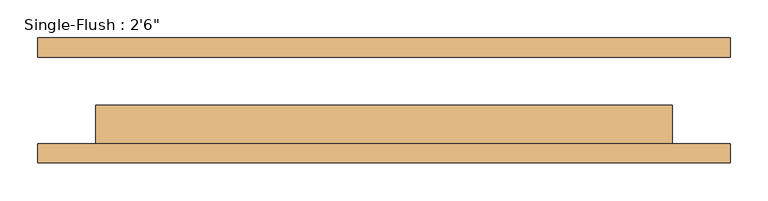
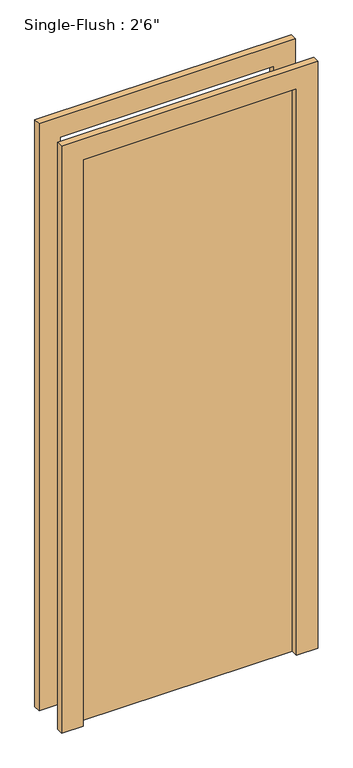
"""IFC4 building model written with IfcOpenShell, lengths in millimetres: door geometry."""

from ifc_helpers import new_model, si_unit, frame, origin, origin_with_axes, place, context, project, spatial, polyline, outline, extrude, source, transform, mapped, element, save


def door_78caadf7(model_context):
    return source(origin(), model_context, "Body", "SweptSolid", [
        extrude(outline(polyline([(2209.8, -457.2), (0.0, -457.2), (0.0, -381.0), (2133.6, -381.0), (2133.6, 381.0), (0.0, 381.0), (0.0, 457.2), (2209.8, 457.2), (2209.8, -457.2)])), frame((0.0, -82.55, 0.0), z_axis=(0.0, 1.0, 0.0), x_axis=(0.0, 0.0, 1.0)), (0.0, 0.0, 1.0), 25.4),
        extrude(outline(polyline([(2209.8, 457.2), (2209.8, -457.2), (0.0, -457.2), (0.0, -381.0), (2133.6, -381.0), (2133.6, 381.0), (0.0, 381.0), (0.0, 457.2), (2209.8, 457.2)])), frame((0.0, 57.15, 0.0), z_axis=(0.0, 1.0, 0.0), x_axis=(0.0, 0.0, 1.0)), (0.0, 0.0, 1.0), 25.4),
        extrude(outline(polyline([(381.0, -6.35), (381.0, -57.15), (-381.0, -57.15), (-381.0, -6.35), (381.0, -6.35)])), origin_with_axes(), (0.0, 0.0, 1.0), 2133.6),
    ])


if __name__ == "__main__":
    model = new_model("IFC4")
    model_context = context("Model", 3, world=origin())
    ifc_project = project(units=[si_unit("LENGTHUNIT", "METRE", prefix="MILLI")], contexts=[model_context])
    site = spatial("IfcSite", under=ifc_project)
    building = spatial("IfcBuilding", under=site)
    placement = place(None, origin())
    door_shape = door_78caadf7(model_context)
    element("IfcDoor", 1, ObjectType="Single-Flush : 2'6\"", at=placement, inside=building, context=model_context, shape_type="MappedRepresentation", body=[
        mapped(door_shape, transform((0.0, 0.0, 0.0), x_axis=(1.0, 0.0, 0.0), y_axis=(0.0, 1.0, 0.0), z_axis=(0.0, 0.0, 1.0))),
    ])
    save(model, "model.ifc")

# Revit data of these elements
# Type "Single-Flush : 2'6\""
#   Type Mark = "10"
#   Construction Type Id = "MDOOR"
#   Assembly Code = "C1020"
#   Analytic Construction = "Metal"
#   Thickness = 0' - 2"
#   Heat Transfer Coefficient (U) = 0.651978 BTU/(h·ft²·°F)
#   Height = 7' - 0"
#   Trim Projection Ext = 0' - 1"
#   Trim Projection Int = 0' - 1"
#   Trim Width = 0' - 3"
#   Width = 2' - 6"
#   Define Thermal Properties by = 1
#   Door Material = Door - Panel
#   Frame Material = Door - Frame
#   Visual Light Transmittance = 0
#   Solar Heat Gain Coefficient = 0
#   Function = (empty or 0)
#   Wall Closure = (empty or 0)
# Element 1 (IfcDoor, "Single-Flush : 2'6\"")
#   Materials on its faces: "Door - Frame", "Door - Panel"
# Materials
#   "Door - Panel": class "Wood", colour RGB 210 159 95, transparency 0, Cost = 0
#   "Door - Frame": colour RGB 118 70 51, transparency 0, Cost = 0
